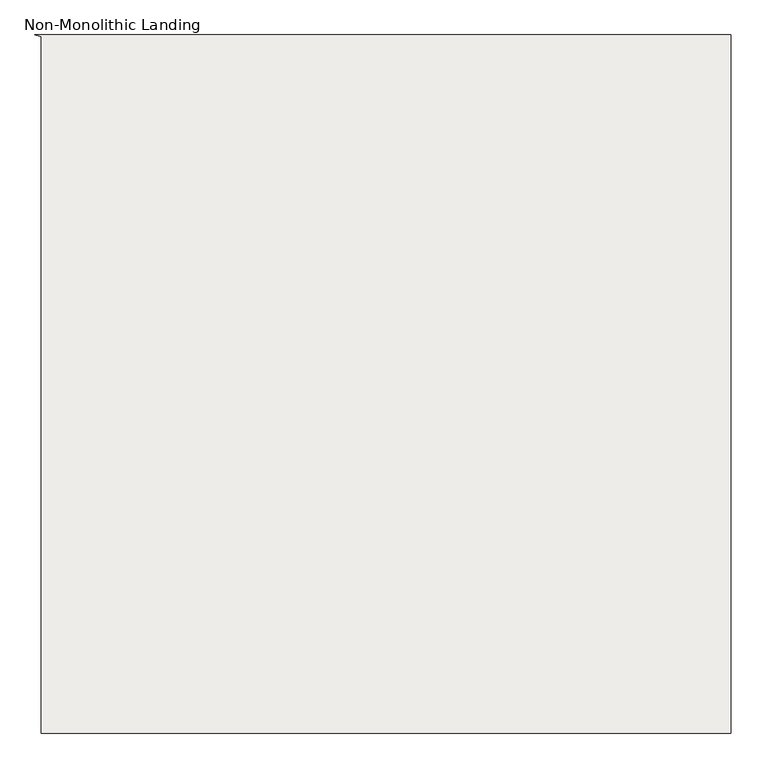
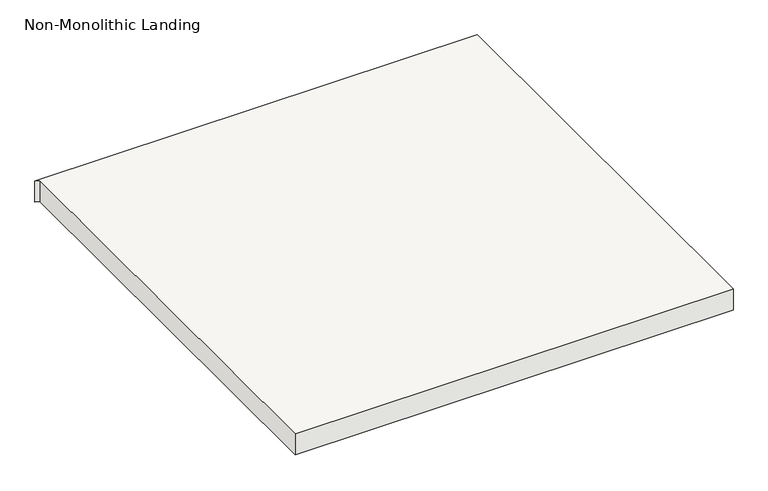
"""IFC4 building model written with IfcOpenShell, lengths in millimetres: slab geometry, Non-Monolithic Landing."""

from ifc_helpers import new_model, si_unit, frame, origin, place, context, project, spatial, polyline, outline, extrude, source, transform, mapped, element, save


def non_monolithic_landing_bd582a30(model_context):
    return source(origin(), model_context, "Body", "SweptSolid", [
        extrude(outline(polyline([(-9477.5794909, -3248.5618509), (-9477.5794909, -4251.1618509), (-10468.1794909, -4251.1618509), (-10468.1794909, -3251.1360696), (-10477.6052721, -3248.5618509), (-9477.5794909, -3248.5618509)])), frame((0.0, 0.0, 5221.2470588), z_axis=(0.0, 0.0, 1.0), x_axis=(1.0, 0.0, 0.0)), (0.0, 0.0, 1.0), 50.0),
    ])


if __name__ == "__main__":
    model = new_model("IFC4")
    model_context = context("Model", 3, world=origin())
    ifc_project = project(units=[si_unit("LENGTHUNIT", "METRE", prefix="MILLI")], contexts=[model_context])
    site = spatial("IfcSite", under=ifc_project)
    building = spatial("IfcBuilding", under=site)
    placement = place(None, origin())
    non_monolithic_landing_shape = non_monolithic_landing_bd582a30(model_context)
    element("IfcSlab", 1, ObjectType="Non-Monolithic Landing", at=placement, inside=building, context=model_context, shape_type="MappedRepresentation", body=[
        mapped(non_monolithic_landing_shape, transform((0.0, 0.0, 0.0), x_axis=(1.0, 0.0, 0.0), y_axis=(0.0, 1.0, 0.0), z_axis=(0.0, 0.0, 1.0))),
    ])
    save(model, "model.ifc")
